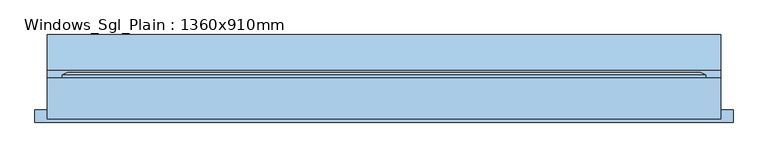
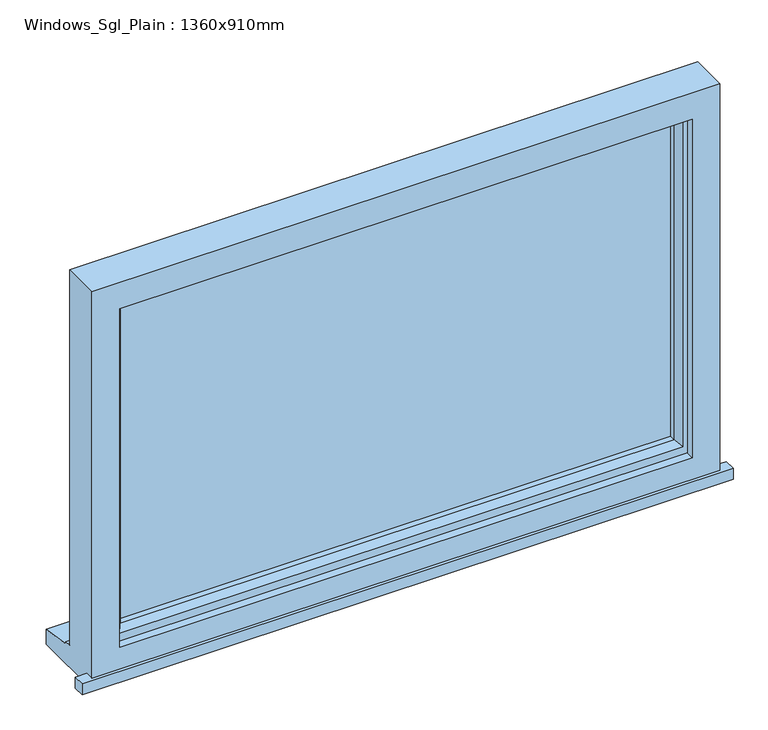
"""IFC4 building model written with IfcOpenShell, lengths in millimetres: window geometry, Windows_Sgl_Plain : 1360x910mm."""

from ifc_helpers import new_model, si_unit, frame, origin, place, context, project, spatial, polyline, outline, extrude, faceted_brep, source, transform, mapped, element, save


def windows_sgl_plain_1360x910mm_1fca1195(model_context):
    return source(origin(), model_context, "Body", "SolidModel", [
        extrude(outline(polyline([(-705.0, -73.6934322), (-705.0, -48.6934322), (-680.0, -48.6934322), (-680.0, -67.3934322), (680.0, -67.3934322), (680.0, -48.6934322), (705.0, -48.6934322), (705.0, -73.6934322), (-705.0, -73.6934322)])), frame((0.0, 0.0, 1200.0), z_axis=(0.0, 0.0, 1.0), x_axis=(1.0, 0.0, 0.0)), (0.0, 0.0, 1.0), 25.0),
        faceted_brep([(-680.0, -67.3934322, 1200.0), (680.0, -67.3934322, 1200.0), (680.0, -67.3934322, 2110.0), (-680.0, -67.3934322, 2110.0), (-620.0, -67.3934322, 2050.0), (620.0, -67.3934322, 2050.0), (620.0, -67.3934322, 1275.0), (-620.0, -67.3934322, 1275.0), (-680.0, 15.6065678, 2110.0), (-680.0, 15.6065678, 1251.0), (-680.0, 30.6065678, 1249.68767), (-680.0, 30.6065678, 1244.7449676), (-680.0, 103.1065678, 1233.8088847), (-680.0, 103.1065678, 1200.0), (680.0, 15.6065678, 2110.0), (680.0, 15.6065678, 1251.0), (-640.0, 15.6065678, 2070.0), (-640.0, 15.6065678, 1263.0), (640.0, 15.6065678, 1263.0), (640.0, 15.6065678, 2070.0), (-640.0, -49.3934322, 2070.0), (-640.0, -49.3934322, 1263.0), (640.0, -49.3934322, 2070.0), (640.0, -49.3934322, 1263.0), (-620.0, -49.3934322, 2050.0), (-620.0, -49.3934322, 1275.0), (620.0, -49.3934322, 1275.0), (620.0, -49.3934322, 2050.0), (680.0, 103.1065678, 1200.0), (680.0, 103.1065678, 1233.8088847), (680.0, 30.6065678, 1244.7449676), (680.0, 30.6065678, 1249.68767)], [[[0, 1, 2, 3], [4, 5, 6, 7]], [[0, 3, 8, 9, 10, 11, 12, 13]], [[9, 8, 14, 15], [16, 17, 18, 19]], [[17, 16, 20, 21]], [[20, 22, 23, 21], [24, 25, 26, 27]], [[24, 4, 7, 25]], [[3, 2, 14, 8]], [[16, 19, 22, 20]], [[5, 4, 24, 27]], [[15, 14, 2, 1, 28, 29, 30, 31]], [[19, 18, 23, 22]], [[5, 27, 26, 6]], [[28, 1, 0, 13]], [[29, 28, 13, 12]], [[30, 29, 12, 11]], [[31, 30, 11, 10]], [[15, 31, 10, 9]], [[21, 23, 18, 17]], [[7, 6, 26, 25]]]),
        extrude(outline(polyline([(610.0, -20.3934322), (-610.0, -20.3934322), (-610.0, 3.6065678), (610.0, 3.6065678), (610.0, -20.3934322)])), frame((0.0, 0.0, 1293.0), z_axis=(0.0, 0.0, 1.0), x_axis=(1.0, 0.0, 0.0)), (0.0, 0.0, 1.0), 747.0),
        faceted_brep([(-650.0, 15.6065678, 2080.0), (-650.0, 21.3800705, 2080.0), (-650.0, 21.3800705, 1253.0), (-650.0, 15.6065678, 1253.0), (-640.0, -49.3934322, 2070.0), (-640.0, 15.6065678, 2070.0), (-640.0, 15.6065678, 1263.0), (-640.0, -49.3934322, 1263.0), (-600.0, -34.9005323, 2030.0), (-610.1480377, -49.3934322, 2040.1480377), (-610.1480377, -49.3934322, 1292.8519623), (-600.0, -34.9005323, 1303.0), (-600.0, -20.3934322, 2030.0), (-600.0, -20.3934322, 1303.0), (-610.0, 3.6065678, 2040.0), (-610.0, -20.3934322, 2040.0), (-610.0, -20.3934322, 1293.0), (-610.0, 3.6065678, 1293.0), (-600.0, 21.3800705, 2030.0), (-600.0, 3.6065678, 2030.0), (-600.0, 3.6065678, 1303.0), (-600.0, 21.3800705, 1303.0), (-617.4457548, 27.1535732, 2047.4457548), (-617.4457548, 27.1535732, 1285.5542452), (-639.2153903, 27.1535732, 2069.2153903), (-639.2153903, 27.1535732, 1263.7846097), (650.0, 21.3800705, 1253.0), (650.0, 15.6065678, 1253.0), (640.0, 15.6065678, 1263.0), (640.0, -49.3934322, 1263.0), (610.1480377, -49.3934322, 1292.8519623), (600.0, -34.9005323, 1303.0), (600.0, -20.3934322, 1303.0), (610.0, -20.3934322, 1293.0), (610.0, 3.6065678, 1293.0), (600.0, 3.6065678, 1303.0), (600.0, 21.3800705, 1303.0), (617.4457548, 27.1535732, 1285.5542452), (639.2153903, 27.1535732, 1263.7846097), (650.0, 21.3800705, 2080.0), (650.0, 15.6065678, 2080.0), (640.0, 15.6065678, 2070.0), (640.0, -49.3934322, 2070.0), (610.1480377, -49.3934322, 2040.1480377), (600.0, -34.9005323, 2030.0), (600.0, -20.3934322, 2030.0), (610.0, -20.3934322, 2040.0), (610.0, 3.6065678, 2040.0), (600.0, 3.6065678, 2030.0), (600.0, 21.3800705, 2030.0), (617.4457548, 27.1535732, 2047.4457548), (639.2153903, 27.1535732, 2069.2153903)], [[[0, 1, 2, 3]], [[4, 5, 6, 7]], [[8, 9, 10, 11]], [[12, 8, 11, 13]], [[14, 15, 16, 17]], [[18, 19, 20, 21]], [[22, 18, 21, 23]], [[1, 24, 25, 2]], [[3, 2, 26, 27]], [[7, 6, 28, 29]], [[11, 10, 30, 31]], [[13, 11, 31, 32]], [[17, 16, 33, 34]], [[21, 20, 35, 36]], [[23, 21, 36, 37]], [[2, 25, 38, 26]], [[27, 26, 39, 40]], [[29, 28, 41, 42]], [[31, 30, 43, 44]], [[32, 31, 44, 45]], [[34, 33, 46, 47]], [[36, 35, 48, 49]], [[37, 36, 49, 50]], [[26, 38, 51, 39]], [[40, 39, 1, 0]], [[3, 27, 40, 0], [5, 41, 28, 6]], [[42, 41, 5, 4]], [[7, 29, 42, 4], [9, 43, 30, 10]], [[44, 43, 9, 8]], [[45, 44, 8, 12]], [[15, 46, 33, 16], [13, 32, 45, 12]], [[47, 46, 15, 14]], [[17, 34, 47, 14], [19, 48, 35, 20]], [[49, 48, 19, 18]], [[50, 49, 18, 22]], [[24, 51, 38, 25], [23, 37, 50, 22]], [[39, 51, 24, 1]]]),
    ])


if __name__ == "__main__":
    model = new_model("IFC4")
    model_context = context("Model", 3, world=origin())
    ifc_project = project(units=[si_unit("LENGTHUNIT", "METRE", prefix="MILLI")], contexts=[model_context])
    site = spatial("IfcSite", under=ifc_project)
    building = spatial("IfcBuilding", under=site)
    placement = place(None, origin())
    windows_sgl_plain_1360x910mm_shape = windows_sgl_plain_1360x910mm_1fca1195(model_context)
    element("IfcWindow", 1, ObjectType="Windows_Sgl_Plain : 1360x910mm", at=placement, inside=building, context=model_context, shape_type="MappedRepresentation", body=[
        mapped(windows_sgl_plain_1360x910mm_shape, transform((0.0, 0.0, 0.0), x_axis=(1.0, 0.0, 0.0), y_axis=(0.0, 1.0, 0.0), z_axis=(0.0, 0.0, 1.0))),
    ])
    save(model, "model.ifc")

# Revit data of these elements
# Type "Windows_Sgl_Plain : 1360x910mm"
#   Type Mark = "46"
#   Operation = "SinglePanel"
#   Construction Type Id = "SGL"
#   Manufacturer = "Revit"
#   Keynote = "L10"
#   Analytic Construction = "Large single-glazed windows"
#   Wrap Layers (Ext) from Ext = 102.5 mm
#   Wrap Layers (Int) from Ext = 177.5 mm
#   Window Board Projection = 25 mm
#   Window Board Extension = 25 mm
#   Visual Light Transmittance = 0.9
#   Solar Heat Gain Coefficient = 0.86
#   Rough Width = 1360 mm
#   Rough Height = 910 mm
#   Height = 910 mm
#   Width = 1360 mm
#   Heat Transfer Coefficient (U) = 5.5617 W/(m²·K)
#   Glazing Thickness = 24 mm
#   FrameOffset - External = 50 mm
#   Frame Depth = 65 mm
#   Default Head Height = 2110 mm
#   Cill Depth = 87.5 mm
#   Cavity Closer Width = 50 mm
#   Cavity Closer Offset from Ext = 102.5 mm
#   Cavity Closer Depth = 85 mm
#   Define Thermal Properties by = 1
#   Vis - Cavity Closers = yes
#   Define Thermal Properties by = 1
#   Material Trim = Window Frame
#   Material Glass = Glass
#   Material Frame = Window Frame
#   Wall Closure = (empty or 0)
# Element 1 (IfcWindow, "Windows_Sgl_Plain : 1360x910mm")
#   Materials on its faces: "Window Frame", "Glass"
# Materials
#   "Window Frame": colour RGB 249 249 249, transparency 0, Keynote = "L10", Cost = 0
#   "Glass": class "Glass", colour RGB 0 128 192, transparency 0.9, Description = "Soda Lime Glass", Cost = 0
